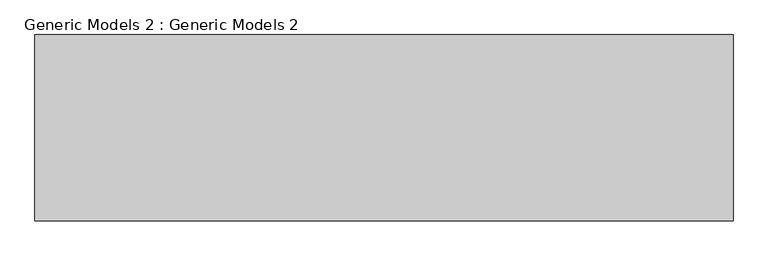
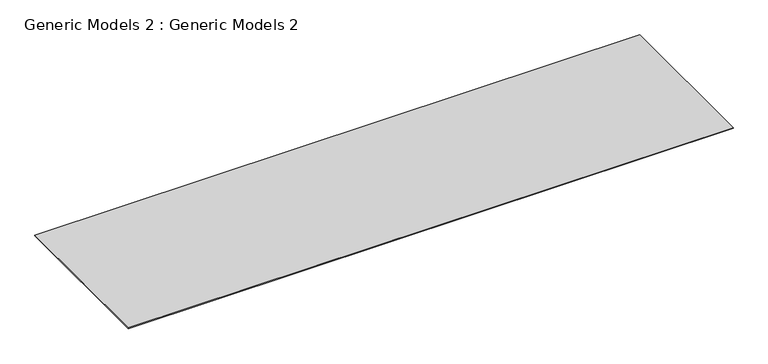
"""IFC4 building model written with IfcOpenShell, lengths in millimetres: proxy geometry, Generic Models 2 : Generic Models 2."""

from ifc_helpers import new_model, si_unit, origin, origin_with_axes, place, context, project, spatial, polyline, outline, extrude, source, transform, mapped, element, save


def generic_models_2_generic_models_2_ab047e66(model_context):
    return source(origin(), model_context, "Body", "SweptSolid", [
        extrude(outline(polyline([(-17326.5657144, 33409.0705427), (19204.5008047, 33409.0705427), (19204.5008047, 23655.4705427), (-17326.5657144, 23655.4705427), (-17326.5657144, 33409.0705427)])), origin_with_axes(), (0.0, 0.0, 1.0), 48.7636508),
    ])


if __name__ == "__main__":
    model = new_model("IFC4")
    model_context = context("Model", 3, world=origin())
    ifc_project = project(units=[si_unit("LENGTHUNIT", "METRE", prefix="MILLI")], contexts=[model_context])
    site = spatial("IfcSite", under=ifc_project)
    building = spatial("IfcBuilding", under=site)
    placement = place(None, origin())
    generic_models_2_generic_models_2_shape = generic_models_2_generic_models_2_ab047e66(model_context)
    element("IfcBuildingElementProxy", 1, Name="Generic Models 2 : Generic Models 2", ObjectType="Generic Models 2 : Generic Models 2", at=placement, inside=building, context=model_context, shape_type="MappedRepresentation", body=[
        mapped(generic_models_2_generic_models_2_shape, transform((0.0, 0.0, 0.0), x_axis=(1.0, 0.0, 0.0), y_axis=(0.0, 1.0, 0.0), z_axis=(0.0, 0.0, 1.0))),
    ])
    save(model, "model.ifc")
